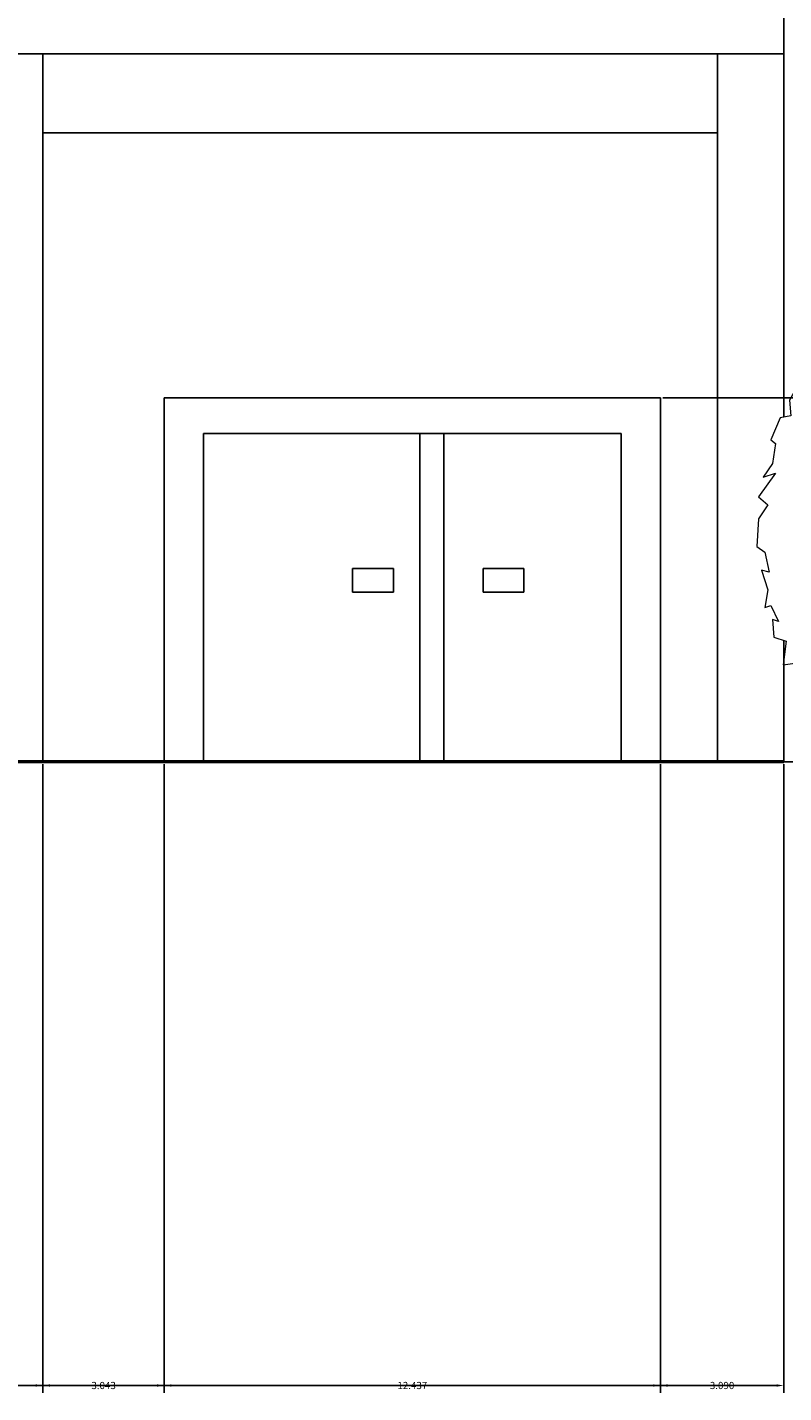
# Model space of a CAD drawing. Units: inches. Extents: x -117 to 121, y -77 to 40.
# Tile 37 of 45: x 72 to 91, y -77 to -43. Entities that reach past the tile are written whole.
import ezdxf

# ---------------------------------------------------------------- set-up
doc = ezdxf.new("R2010")
doc.units = ezdxf.units.IN
doc.header["$MEASUREMENT"] = 0
for name, color, linetype, lineweight in [('A-ANNO-DIMS', 2, 'Continuous', 18), ('A-ELEV', 7, 'Continuous', 25), ('A-ELEV-GRND', 7, 'Continuous', 50), ('L-PLNT', 3, 'Continuous', 13)]:
    doc.layers.add(name, color=color, linetype=linetype, lineweight=lineweight)
doc.styles.get("Standard").update_dxf_attribs({"font": 'arial.ttf'})
doc.dimstyles.get("Standard").update_dxf_attribs({"dimtxt": 0.18, "dimasz": 0.18, "dimexe": 0.18, "dimexo": 0.0625, "dimgap": 0.09, "dimtad": 0, "dimtih": 1, "dimtoh": 1, "dimdec": 4, "dimzin": 0, "dimdsep": 46, "dimtxsty": 'Standard', "dimcen": 0.09, "dimadec": 0, "dimazin": 0, "dimtfac": 1, "dimtdec": 4, "dimtofl": 0, "dimtmove": 0, "dimatfit": 3, "dimfxl": 1, "dimtolj": 1, "dimtzin": 0, "dimarcsym": 0})

# ---------------------------------------------------------------- blocks, each defined once
blk = doc.blocks.new('*U2')
blk.add_lwpolyline([(-2.754, 191.699), (-6.78, 182.851), (-13.682, 176.953), (-11.956, 173.266), (-9.656, 172.529), (-14.257, 170.317), (-13.682, 167.368), (-21.733, 157.783), (-25.184, 154.834), (-21.158, 150.41), (-21.733, 147.461), (-22.884, 140.825), (-26.334, 140.087), (-29.21, 134.926), (-28.635, 129.028), (-32.661, 128.291), (-36.111, 120.18), (-34.386, 118.706), (-35.536, 111.333), (-38.987, 106.171), (-34.386, 107.646), (-40.712, 98.798), (-37.261, 95.849), (-40.712, 90.688), (-41.287, 80.366), (-38.412, 78.154), (-36.686, 70.781), (-39.562, 71.518), (-37.261, 64.145), (-38.412, 57.509), (-36.111, 58.247), (-33.236, 52.348), (-35.536, 53.086), (-34.961, 46.45), (-30.36, 44.975), (-31.51, 36.128), (-26.334, 36.865), (-23.459, 39.814), (-18.283, 36.128), (-20.008, 33.178), (-14.832, 31.704), (-11.956, 33.178), (-12.531, 27.28), (-6.205, 22.856), (-3.905, 24.331), (0.121, 22.856), (8.173, 26.543), (11.624, 25.068), (12.199, 27.28), (21.4, 34.653), (19.675, 39.077), (23.701, 44.975), (30.027, 47.924), (30.602, 53.823), (25.426, 56.772), (32.903, 61.196), (34.053, 67.094), (30.602, 75.205), (34.628, 89.951), (26.576, 103.222), (23.701, 103.222), (28.302, 107.646), (23.701, 110.595), (26.576, 115.756), (25.426, 117.968), (20.825, 118.706), (24.276, 124.604), (22.551, 137.876), (19.1, 139.35), (22.551, 140.825), (19.675, 151.884), (14.499, 153.359), (16.224, 162.207), (12.199, 170.317), (10.473, 167.368), (5.872, 179.165), (4.147, 177.69), (0.696, 187.275), (-0.454, 185.8)], close=True)
for points in [[(-6.813, 23.669), (-6.813, 11.669), (-8.627, 0)], [(0.387, 23.669), (-0.576, 13.271), (-0.576, 3.686), (0, 0)]]:
    blk.add_lwpolyline(points)
blk = doc.blocks.new('*D7')
at = {"layer": 'A-ANNO-DIMS', "color": 0, "lineweight": -2, "transparency": 16777216}
for p, q in [((-77.763, -61.431), (-77.763, -77.193)), ((90.549, -61.438), (90.549, -77.193)), ((-77.583, -77.013), (6.008, -77.013)), ((90.369, -77.013), (6.778, -77.013))]:
    blk.add_line(p, q, dxfattribs=at)
at = {"layer": 'A-ANNO-DIMS', "color": 0, "transparency": 16777216}
for points in [[(-77.583, -76.983), (-77.583, -77.043), (-77.763, -77.013)], [(90.369, -76.983), (90.369, -77.043), (90.549, -77.013)]]:
    blk.add_solid(points, dxfattribs=at)
at = {"layer": 'Defpoints', "color": 0, "transparency": 16777216}
for p in [(-77.763, -61.369), (90.549, -61.376), (90.549, -77.013)]:
    blk.add_point(p, dxfattribs=at)
at = {"layer": 'A-ANNO-DIMS', "color": 0, "transparency": 16777216, "insert": (6.393, -77.013), "char_height": 0.18, "attachment_point": 5}
blk.add_mtext('\\A1;168.3', dxfattribs=at)
blk = doc.blocks.new('*D24')
at = {"layer": 'A-ANNO-DIMS', "color": 0, "lineweight": -2, "transparency": 16777216}
for p, q in [((87.242, 3.166), (87.242, 38.61)), ((87.422, 38.43), (98.081, 38.43)), ((109.67, 38.43), (99.011, 38.43)), ((109.85, -61.313), (109.85, 38.61))]:
    blk.add_line(p, q, dxfattribs=at)
at = {"layer": 'A-ANNO-DIMS', "color": 0, "transparency": 16777216}
for points in [[(87.422, 38.46), (87.422, 38.4), (87.242, 38.43)], [(109.67, 38.46), (109.67, 38.4), (109.85, 38.43)]]:
    blk.add_solid(points, dxfattribs=at)
at = {"layer": 'Defpoints', "color": 0, "transparency": 16777216}
for p in [(109.85, 38.43), (87.242, 3.104), (109.85, -61.376)]:
    blk.add_point(p, dxfattribs=at)
at = {"layer": 'A-ANNO-DIMS', "color": 0, "transparency": 16777216, "insert": (98.546, 38.43), "char_height": 0.18, "attachment_point": 5}
blk.add_mtext('\\A1;22.609', dxfattribs=at)
blk = doc.blocks.new('*D28')
at = {"layer": 'A-ANNO-DIMS', "color": 0, "lineweight": -2, "transparency": 16777216}
for p, q in [((54.542, -61.438), (54.542, -77.193)), ((71.979, -61.438), (71.979, -77.193)), ((54.722, -77.013), (62.805, -77.013)), ((71.799, -77.013), (63.716, -77.013))]:
    blk.add_line(p, q, dxfattribs=at)
at = {"layer": 'A-ANNO-DIMS', "color": 0, "transparency": 16777216}
for points in [[(54.722, -76.983), (54.722, -77.043), (54.542, -77.013)], [(71.799, -76.983), (71.799, -77.043), (71.979, -77.013)]]:
    blk.add_solid(points, dxfattribs=at)
at = {"layer": 'Defpoints', "color": 0, "transparency": 16777216}
for p in [(54.542, -61.376), (71.979, -61.376), (71.979, -77.013)]:
    blk.add_point(p, dxfattribs=at)
at = {"layer": 'A-ANNO-DIMS', "color": 0, "transparency": 16777216, "insert": (63.261, -77.013), "char_height": 0.18, "attachment_point": 5}
blk.add_mtext('\\A1;17.437', dxfattribs=at)
blk = doc.blocks.new('*D29')
at = {"layer": 'A-ANNO-DIMS', "color": 0, "lineweight": -2, "transparency": 16777216}
for p, q in [((71.979, -61.438), (71.979, -77.193)), ((75.022, -61.438), (75.022, -77.193)), ((72.159, -77.013), (73.107, -77.013)), ((74.842, -77.013), (73.894, -77.013))]:
    blk.add_line(p, q, dxfattribs=at)
at = {"layer": 'A-ANNO-DIMS', "color": 0, "transparency": 16777216}
for points in [[(72.159, -76.983), (72.159, -77.043), (71.979, -77.013)], [(74.842, -76.983), (74.842, -77.043), (75.022, -77.013)]]:
    blk.add_solid(points, dxfattribs=at)
at = {"layer": 'Defpoints', "color": 0, "transparency": 16777216}
for p in [(71.979, -61.376), (75.022, -61.376), (75.022, -77.013)]:
    blk.add_point(p, dxfattribs=at)
at = {"layer": 'A-ANNO-DIMS', "color": 0, "transparency": 16777216, "insert": (73.501, -77.013), "char_height": 0.18, "attachment_point": 5}
blk.add_mtext('\\A1;3.043', dxfattribs=at)
blk = doc.blocks.new('*D30')
at = {"layer": 'A-ANNO-DIMS', "color": 0, "lineweight": -2, "transparency": 16777216}
for p, q in [((75.022, -61.438), (75.022, -77.193)), ((87.459, -61.438), (87.459, -77.193)), ((75.202, -77.013), (80.785, -77.013)), ((87.279, -77.013), (81.695, -77.013))]:
    blk.add_line(p, q, dxfattribs=at)
at = {"layer": 'A-ANNO-DIMS', "color": 0, "transparency": 16777216}
for points in [[(75.202, -76.983), (75.202, -77.043), (75.022, -77.013)], [(87.279, -76.983), (87.279, -77.043), (87.459, -77.013)]]:
    blk.add_solid(points, dxfattribs=at)
at = {"layer": 'Defpoints', "color": 0, "transparency": 16777216}
for p in [(75.022, -61.376), (87.459, -61.376), (87.459, -77.013)]:
    blk.add_point(p, dxfattribs=at)
at = {"layer": 'A-ANNO-DIMS', "color": 0, "transparency": 16777216, "insert": (81.24, -77.013), "char_height": 0.18, "attachment_point": 5}
blk.add_mtext('\\A1;12.437', dxfattribs=at)
blk = doc.blocks.new('*D31')
at = {"layer": 'A-ANNO-DIMS', "color": 0, "lineweight": -2, "transparency": 16777216}
for p, q in [((87.459, -61.438), (87.459, -77.193)), ((90.549, -61.438), (90.549, -77.193)), ((87.639, -77.013), (88.61, -77.013)), ((90.369, -77.013), (89.397, -77.013))]:
    blk.add_line(p, q, dxfattribs=at)
at = {"layer": 'A-ANNO-DIMS', "color": 0, "transparency": 16777216}
for points in [[(87.639, -76.983), (87.639, -77.043), (87.459, -77.013)], [(90.369, -76.983), (90.369, -77.043), (90.549, -77.013)]]:
    blk.add_solid(points, dxfattribs=at)
at = {"layer": 'Defpoints', "color": 0, "transparency": 16777216}
for p in [(87.459, -61.376), (90.549, -61.376), (90.549, -77.013)]:
    blk.add_point(p, dxfattribs=at)
at = {"layer": 'A-ANNO-DIMS', "color": 0, "transparency": 16777216, "insert": (89.004, -77.013), "char_height": 0.18, "attachment_point": 5}
blk.add_mtext('\\A1;3.090', dxfattribs=at)
blk = doc.blocks.new('*D38')
at = {"layer": 'A-ANNO-DIMS', "color": 0, "lineweight": -2, "transparency": 16777216}
for p, q in [((87.521, -52.254), (120.84, -52.254)), ((120.66, -52.434), (120.66, -56.633)), ((120.66, -61.196), (120.66, -56.997)), ((87.521, -61.376), (120.84, -61.376))]:
    blk.add_line(p, q, dxfattribs=at)
at = {"layer": 'A-ANNO-DIMS', "color": 0, "transparency": 16777216}
for points in [[(120.63, -52.434), (120.69, -52.434), (120.66, -52.254)], [(120.63, -61.196), (120.69, -61.196), (120.66, -61.376)]]:
    blk.add_solid(points, dxfattribs=at)
at = {"layer": 'Defpoints', "color": 0, "transparency": 16777216}
for p in [(87.459, -52.254), (87.459, -61.376), (120.66, -61.376)]:
    blk.add_point(p, dxfattribs=at)
at = {"layer": 'A-ANNO-DIMS', "color": 0, "transparency": 16777216, "insert": (120.66, -56.815), "char_height": 0.18, "attachment_point": 5}
blk.add_mtext('\\A1;9.122', dxfattribs=at)

msp = doc.modelspace()

# ---------------------------------------------------------------- linework, layer by layer
at = {"layer": 'A-ELEV'}
for p, q in [((90.5486, -44.5456), (90.5486, -41.7053)), ((70.6214, -43.6334), (90.5486, -43.6334)), ((71.9791, -61.3756), (71.9791, -43.6334)), ((88.8877, -61.3756), (88.8877, -43.6334)), ((90.5486, -44.5456), (90.5486, -52.7421)), ((71.9791, -45.6125), (88.8877, -45.6125)), ((75.022, -61.3756), (75.022, -52.2539)), ((75.022, -52.2539), (87.4587, -52.2539)), ((87.4587, -52.2539), (87.4587, -61.3756)), ((76.0062, -61.3756), (76.0062, -53.1476)), ((76.0062, -53.1476), (86.4745, -53.1476)), ((81.4275, -61.3756), (81.4275, -53.1476)), ((82.0258, -61.3756), (82.0258, -53.1476)), ((86.4745, -61.3756), (86.4745, -53.1476)), ((79.7436, -56.5311), (80.7642, -56.5311)), ((79.7436, -57.1287), (79.7436, -56.5311)), ((80.7642, -56.5311), (80.7642, -57.1287)), ((83.0167, -56.5311), (84.0374, -56.5311)), ((83.0167, -57.1287), (83.0167, -56.5311)), ((84.0374, -56.5311), (84.0374, -57.1287)), ((80.7642, -57.1287), (79.7436, -57.1287)), ((84.0374, -57.1287), (83.0167, -57.1287)), ((90.5486, -58.3338), (90.5486, -61.3756)), ((90.5486, -61.3756), (88.8877, -61.3756)), ((90.5486, -61.3756), (109.8502, -61.3756))]:
    msp.add_line(p, q, dxfattribs=at)
at = {"layer": 'A-ELEV-GRND'}
msp.add_line((90.5486, -61.3756), (-87.9273, -61.3756), dxfattribs=at)

# ---------------------------------------------------------------- block references
at = {"layer": 'L-PLNT', "xscale": 0.0671647796176818, "yscale": 0.0671647796176818, "zscale": 0.0671647796176818}
msp.add_blockref('*U2', (92.6522, -61.3752), dxfattribs=at)

# ---------------------------------------------------------------- dimensions: what is measured, and where the dimension line sits
at = {"layer": 'A-ANNO-DIMS'}
for base, p1, p2, override, picture, middle in [((109.8502, 38.4297), (87.2416, 3.1036), (109.8502, -61.3756), {"dimdec": 3, "dimlfac": 1, "dimrnd": 0, "dimzin": 0, "dimdsep": 46, "dimlunit": 2}, '*D24', (98.5459, 38.4297)), ((90.5486, -77.0135), (-77.7631, -61.3689), (90.5486, -61.3756), {"dimdec": 1, "dimlfac": 1, "dimrnd": 0, "dimzin": 0, "dimdsep": 46, "dimlunit": 2}, '*D7', (6.3928, -77.0135)), ((71.9791, -77.0135), (54.5419, -61.3756), (71.9791, -61.3756), {"dimdec": 3, "dimlfac": 1, "dimrnd": 0, "dimzin": 0, "dimdsep": 46, "dimlunit": 2}, '*D28', (63.2605, -77.0135)), ((75.022, -77.0135), (71.9791, -61.3756), (75.022, -61.3756), {"dimdec": 3, "dimlfac": 1, "dimrnd": 0, "dimzin": 0, "dimdsep": 46, "dimlunit": 2}, '*D29', (73.5006, -77.0135)), ((87.4587, -77.0135), (75.022, -61.3756), (87.4587, -61.3756), {"dimdec": 3, "dimlfac": 1, "dimrnd": 0, "dimzin": 0, "dimdsep": 46, "dimlunit": 2}, '*D30', (81.2403, -77.0135)), ((90.5486, -77.0135), (87.4587, -61.3756), (90.5486, -61.3756), {"dimdec": 3, "dimlfac": 1, "dimrnd": 0, "dimzin": 0, "dimdsep": 46, "dimlunit": 2}, '*D31', (89.0036, -77.0135))]:
    dim = msp.add_linear_dim(base=base, p1=p1, p2=p2, dimstyle='Standard', override=override, dxfattribs=at)
    dim.commit()
    dim.dimension.update_dxf_attribs({"geometry": picture, "text_midpoint": middle})
dim = msp.add_linear_dim(base=(120.6602, -61.3756), p1=(87.4587, -52.2539), p2=(87.4587, -61.3756), angle=90, dimstyle='Standard', override={"dimdec": 3, "dimlfac": 1, "dimrnd": 0, "dimzin": 0, "dimdsep": 46, "dimlunit": 2}, dxfattribs=at)
dim.commit()
dim.dimension.update_dxf_attribs({"geometry": '*D38', "text_midpoint": (120.6602, -56.8148)})

doc.saveas('drawing.dxf')
